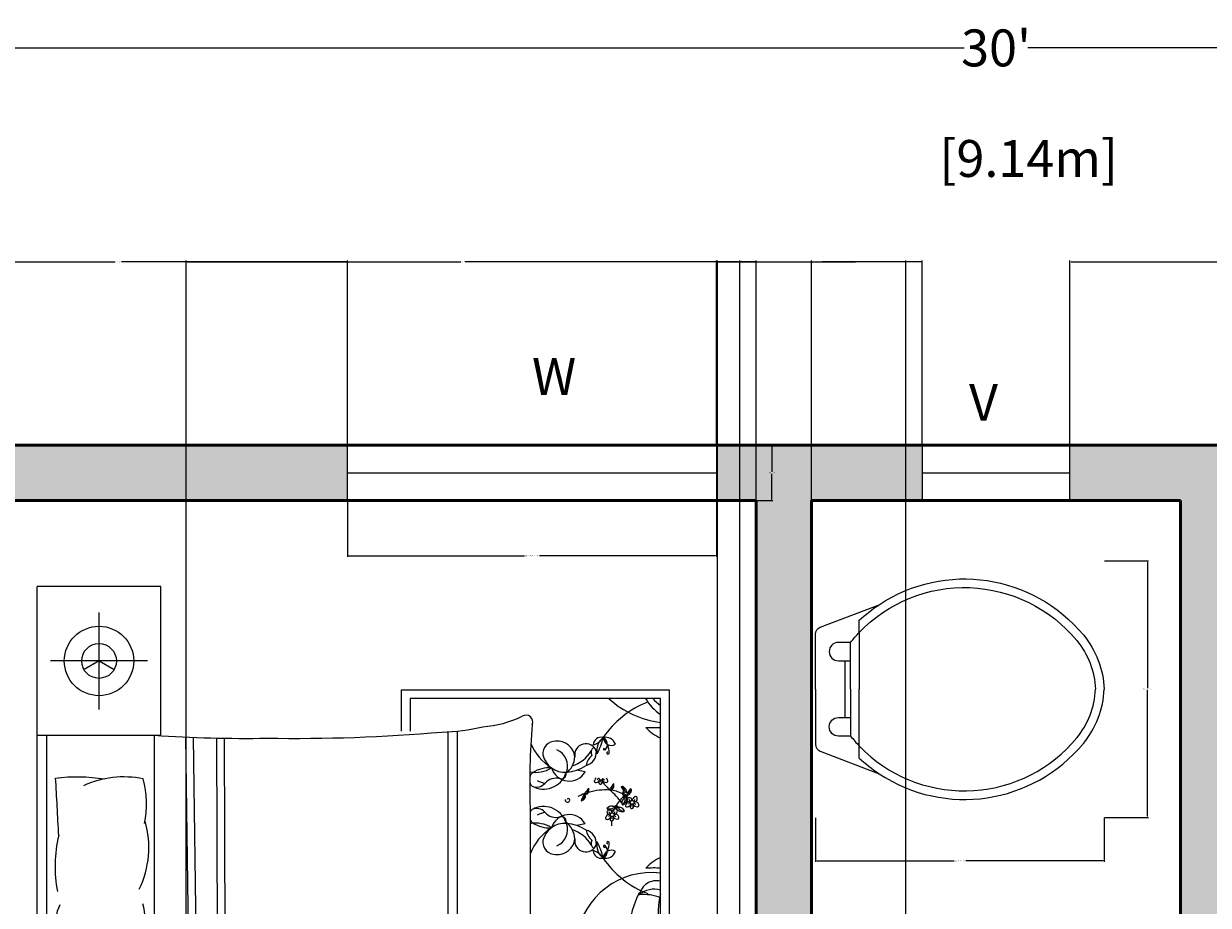
# Model space of a CAD drawing. Units: inches. Extents: x -55 to 413, y -498 to 86.
# Tile 5 of 6: x 45 to 238, y -57 to 86. Entities that reach past the tile are written whole.
import ezdxf

# ---------------------------------------------------------------- set-up
doc = ezdxf.new("R2010")
doc.units = ezdxf.units.IN
doc.header["$MEASUREMENT"] = 0
for name, color, linetype, lineweight in [('A-ANNO-DIMS', 2, 'Continuous', 18), ('A-ANNO-TEXT', 7, 'Continuous', 25), ('A-FLOR-FIXT', 9, 'Continuous', 18), ('A-FURN', 9, 'Continuous', 18), ('A-GLAZ', 4, 'Continuous', 18), ('A-WALL', 7, 'Continuous', 50), ('A-WALL-PATT', 8, 'Continuous', 13)]:
    doc.layers.add(name, color=color, linetype=linetype, lineweight=lineweight)
doc.styles.get("Standard").update_dxf_attribs({"font": 'arial.ttf'})
doc.dimstyles.get("Standard").update_dxf_attribs({"dimtxt": 0.18, "dimasz": 0.18, "dimexe": 0.18, "dimexo": 0.0625, "dimgap": 0.09, "dimtad": 0, "dimtih": 1, "dimtoh": 1, "dimdec": 0, "dimzin": 0, "dimdsep": 46, "dimlunit": 3, "dimtxsty": 'Standard', "dimcen": 0.09, "dimadec": 0, "dimazin": 0, "dimtfac": 1, "dimtdec": 0, "dimtofl": 0, "dimtmove": 0, "dimatfit": 3, "dimfxl": 1, "dimtolj": 1, "dimtzin": 0, "dimarcsym": 0})

# ---------------------------------------------------------------- blocks, each defined once
blk = doc.blocks.new('*D2')
at = {"layer": 'A-ANNO-DIMS', "color": 0, "lineweight": -2, "transparency": 16777216}
for p, q in [((23, 17.6), (23, 82.27)), ((23.18, 82.09), (197.82, 82.09)), ((382.82, 82.09), (208.18, 82.09)), ((383, 17.6), (383, 82.27))]:
    blk.add_line(p, q, dxfattribs=at)
at = {"layer": 'A-ANNO-DIMS', "color": 0, "transparency": 16777216}
for points in [[(23.18, 82.12), (23.18, 82.06), (23, 82.09)], [(382.82, 82.12), (382.82, 82.06), (383, 82.09)]]:
    blk.add_solid(points, dxfattribs=at)
at = {"layer": 'Defpoints', "color": 0, "transparency": 16777216}
for p in [(383, 82.09), (23, 17.54), (383, 17.54)]:
    blk.add_point(p, dxfattribs=at)
at = {"layer": 'A-ANNO-DIMS', "color": 0, "transparency": 16777216, "insert": (203, 82.09), "char_height": 6, "attachment_point": 5}
blk.add_mtext("\\A1;30'", dxfattribs=at)
blk = doc.blocks.new('BED-DOUBLE-WITH-NIGHTSTANDS')
for p, q in [((0, 0), (0, 120.84)), ((10.07, 100.86), (10.07, 116.65)), ((17.96, 108.75), (2.18, 108.75)), ((59.24, 97.34), (59.24, 104.05)), ((59.24, 104.05), (102.77, 104.05)), ((102.77, 104.05), (102.77, 15.95)), ((60.64, 102.65), (60.64, 97.32)), ((101.37, 102.65), (60.64, 102.65)), ((101.37, 17.35), (101.37, 102.65)), ((1.55, 96.67), (1.55, 24.17)), ((19.1, 24.17), (19.1, 96.67)), ((24.12, 96.35), (24.72, 53.32)), ((25.36, 96.3), (25.98, 52.42)), ((66.77, 97.22), (66.77, 22.78)), ((68.28, 97.33), (68.28, 22.78)), ((29.16, 96.24), (29.34, 50.35)), ((30.4, 96.24), (30.59, 49.88)), ((89.11, 90.74), (87.75, 91)), ((80.15, 84.95), (80.15, 35.89)), ((89.11, 82.29), (87.75, 82.03)), ((19.1, 57.36), (28.31, 50.74)), ((22.69, 40.95), (19.1, 54.13)), ((28.31, 50.74), (35.41, 48.05)), ((35.41, 48.05), (38.59, 47.56)), ((38.59, 47.56), (37.61, 43.64)), ((37.61, 43.64), (36.14, 40.46)), ((25.87, 32.14), (22.69, 40.95)), ((36.14, 40.46), (35.41, 35.08)), ((89.11, 37.7), (87.75, 37.97)), ((35.41, 35.08), (34.92, 28.96)), ((29.29, 27.49), (25.87, 32.14)), ((34.92, 28.96), (35.41, 24.06)), ((89.11, 29.26), (87.75, 28.99)), ((34.43, 23.09), (29.29, 27.49)), ((0, 24.17), (33.17, 24.17)), ((35.41, 24.06), (34.43, 23.09)), ((59.24, 15.95), (59.24, 22.78)), ((60.64, 22.78), (60.64, 17.35)), ((10.07, 19.98), (10.07, 4.19)), ((60.64, 17.35), (101.37, 17.35)), ((102.77, 15.95), (59.24, 15.95)), ((17.96, 12.08), (2.18, 12.08))]:
    blk.add_line(p, q)
for points in [[(0, 96.67), (20.14, 96.67), (20.14, 120.84), (0, 120.84)], [(10.07, 108.75), (7.63, 107.35)], [(10.07, 108.75), (12.51, 107.35)], [(20.14, 24.17), (20.14, 0), (0, 0)], [(10.07, 12.08), (7.63, 13.49)], [(10.07, 12.08), (12.51, 13.49)]]:
    blk.add_lwpolyline(points)
for points in [[(65.82, 97.19, 0.056112), (72.47, 98.06, 0.095341), (78.87, 99.76)], [(3.01, 89.73, -0.074897), (10.9, 89.58, 0.472817)], [(11.35, 65.01, -0.14099), (3.29, 64.77, -0.235245)], [(11.35, 59.85, 0.14099), (3.29, 60.09, 0.235245)], [(3.01, 31.11, 0.074897), (10.9, 31.25, -0.472817)], [(45.49, 22.83, 0.001242), (68.42, 22.78, -0.127202), (79.85, 20.35)]]:
    blk.add_lwpolyline(points, format="xyb")
for centre, radius in [((10.07, 108.75), 5.64), ((10.07, 108.75), 2.82), ((96.74, 85.77), 0.308), ((93.49, 83.76), 0.308), ((93.49, 36.24), 0.308), ((96.74, 34.23), 0.308), ((10.07, 12.08), 5.64), ((10.07, 12.08), 2.82)]:
    blk.add_circle(centre, radius)
for centre, radius, start, end in [((105.05, 87.4), 15.78, 111.4092, 145.6135), ((103.49, 114.39), 15.78, 228.1144, 262.255), ((105.6, 106.48), 7.69, 209.8884, 236.5383), ((107.04, 109.24), 9.58, 223.5186, 233.6964), ((79.49, 98.85), 1.1, 336.5219, 123.8264), ((197.68, 88.65), 117.59, 175.2402, 181.8035), ((33.86, 313.3), 217.13, 266.1, 270.9282), ((41.76, 379.4), 283.23, 269.1145, 274.8735), ((91.72, 95.04), 1.31, 76.272, 177.0484), ((89.73, 97.71), 2.7, 284.7031, 328.6173), ((93.49, 94.28), 2.49, 125.7657, 194.5347), ((81.25, 98.7), 11.04, 332.8176, 347.4827), ((92.4, 94.6), 1.75, 20.9613, 102.2885), ((93.35, 96.35), 1.32, 181.7131, 301.5367), ((89.03, 93.68), 3.99, 2.0648, 41.1598), ((91.43, 95.17), 1.29, 316.2238, 62.3173), ((103.83, 102.17), 6.42, 221.0454, 247.4453), ((100.38, 119.75), 21.83, 266.3481, 272.5919), ((88.66, 99), 9.15, 203.6453, 236.3329), ((84.27, 93.67), 2.04, 88.9462, 185.5144), ((84.56, 92.84), 2.89, 7.1143, 95.0551), ((89.21, 93.5), 1.81, 19.1312, 189.736), ((91.18, 93.88), 1.11, 126.7319, 206.0245), ((92.17, 94.41), 0.103, 20.2667, 316.2271), ((85.78, 94.3), 3.63, 193.079, 274.7067), ((83.46, 91.7), 2.8, 338.5779, 68.4181), ((83.92, 93.34), 3.51, 305.9599, 357.6409), ((85.22, 97.1), 5.7, 288.2955, 328.7386), ((88.67, 93.94), 2.26, 285.6955, 4.031), ((91.68, 91.5), 2.41, 128.4175, 173.8338), ((92.82, 93.82), 0.196, 168.5166, 2.0648), ((92.72, 93.84), 0.0952, 52.0591, 168.5166), ((81.49, 89.45), 1.46, 127.675, 162.5814), ((81.04, 95.65), 5.01, 259.249, 301.1782), ((83.22, 86.74), 4.66, 85.2696, 124.215), ((86.51, 92.24), 3, 196.8663, 330.0915), ((83.22, 86.74), 4.66, 53.6555, 57.2989), ((85.68, 97.15), 6.48, 273.4924, 303.7117), ((-1146.98, 23.12), 1151.92, 2.85022, 3.31479), ((14.07, 74.34), 15.57, 78.2417, 114.8684), ((1.6, 85.42), 16.19, 348.9631, 14.8961), ((81.49, 89.45), 1.46, 196.6343, 225.5483), ((82.34, 91.77), 3.85, 240.8249, 340.7178), ((81.2, 90.06), 1.81, 246.1646, 318.4347), ((83.04, 92.35), 3.47, 240.0851, 262.564), ((84.4, 87.22), 2.48, 74.8529, 138.4347), ((85.25, 90.33), 0.75, 254.8529, 12.6959), ((90.82, 89.21), 0.238, 125.0752, 284.7644), ((91.19, 89.3), 0.513, 127.3642, 168.4363), ((90.79, 89.71), 0.74, 277.4968, 341.2737), ((91.37, 89.36), 0.294, 88.1325, 178.8919), ((91.96, 89.05), 0.636, 136.3462, 189.6513), ((91.6, 88.99), 0.265, 189.6513, 312.3208), ((91.66, 89.72), 0.308, 183.2768, 356.7232), ((92.63, 89.17), 1.01, 164.2829, 186.9148), ((91.44, 89.17), 0.504, 312.3208, 40.2111), ((92.5, 89.73), 0.715, 201.6382, 274.947), ((91.56, 88.75), 0.934, 42.3896, 66.5724), ((100.98, 96.15), 11.47, 217.9541, 226.8459), ((92.23, 89.3), 0.508, 10.9597, 52.2379), ((92.55, 89.26), 0.236, 274.947, 37.5263), ((94.05, 88.22), 0.634, 115.5379, 168.6744), ((91.9, 89.14), 1.91, 329.344, 349.7412), ((90.37, 88.7), 3.41, 352.8698, 1.6736), ((92.47, 77.79), 10.01, 110.1059, 116.9968), ((86.93, 87.31), 1.94, 336.3901, 344.4871), ((89.04, 86.81), 0.246, 83.9457, 185.6216), ((88.06, 87.04), 1.01, 328.836, 0.8141), ((88.58, 86.75), 0.58, 306.5232, 32.4668), ((89.27, 87.2), 0.246, 112.5583, 214.2343), ((89.11, 87.64), 0.58, 265.7131, 351.6568), ((88.6, 87.96), 1.01, 297.3659, 329.344), ((87.84, 88.83), 1.94, 313.6929, 321.7899), ((89.98, 87.5), 0.634, 115.5379, 168.6744), ((87.83, 88.42), 1.91, 329.344, 349.7412), ((92.47, 77.79), 10.01, 86.1723, 106.4158), ((86.31, 87.98), 3.41, 352.8698, 1.6736), ((93.34, 87.92), 0.246, 112.5583, 214.2343), ((93.18, 88.36), 0.58, 265.7131, 351.6568), ((92.67, 88.68), 1.01, 297.3659, 329.344), ((92.72, 82.78), 5.02, 60.7959, 85.244), ((82.04, 75.56), 16.51, 37.8256, 47.7588), ((91.9, 89.55), 1.94, 313.6929, 321.7899), ((99.38, 82.26), 6.02, 130.182, 149.456), ((95.16, 88.01), 0.344, 33.0979, 123.1364), ((87.59, 83.16), 8.99, 31.1156, 34.8118), ((94.67, 87.42), 0.93, 2.3172, 70.5201), ((94.22, 86.41), 1.4, 310.9365, 22.7695), ((95.43, 87.19), 0.268, 135.7354, 318.1297), ((94.99, 87.63), 0.356, 315.7354, 31.1156), ((94.69, 86.87), 0.826, 319.3812, 5.5456), ((95.64, 87.19), 0.268, 68.2452, 250.6395), ((95.02, 87.52), 0.801, 352.6008, 57.1845), ((97.88, 82.14), 5.36, 111.7087, 116.2181), ((92.72, 82.78), 5.02, 47.5083, 55.9967), ((95.78, 87.7), 0.801, 252.8042, 349.6943), ((95.02, 86.27), 0.853, 331.1838, 51.6792), ((95.87, 87.77), 0.356, 248.2452, 323.6254), ((95.55, 87.99), 0.93, 291.7087, 3.0299), ((88.91, 92.89), 8.99, 323.6254, 327.3216), ((96.29, 87.75), 0.344, 325.6077, 55.6462), ((97.67, 85.85), 0.97, 121.9501, 165.2442), ((97.31, 86.42), 0.305, 44.3732, 121.9501), ((82.34, 81.26), 3.85, 19.2822, 119.1751), ((81.2, 82.97), 1.81, 41.5653, 113.8354), ((86.24, 86.19), 0.379, 169.5864, 349.5616), ((86.38, 86.17), 0.233, 349.5616, 167.2949), ((89.11, 86.04), 0.634, 129.5056, 182.6421), ((87.29, 87.51), 1.91, 308.4388, 328.836), ((86.96, 89.06), 3.41, 296.5064, 305.3102), ((93.04, 86.11), 1.4, 253.6301, 325.4631), ((93.43, 84.17), 0.992, 82.0748, 142.6895), ((93.32, 85.53), 1.02, 228.342, 274.9894), ((93.35, 85.36), 0.853, 273.8774, 357.1501), ((93.68, 85.97), 0.826, 262.0748, 308.2393), ((95.01, 85.12), 0.853, 181.4625, 249.4747), ((94.87, 85.79), 0.826, 215.1128, 261.2773), ((95.53, 85.75), 1.4, 197.889, 269.722), ((94.59, 84), 0.992, 20.6625, 81.2773), ((96.07, 85.69), 0.992, 139.3812, 199.9959), ((94.86, 86.33), 1.02, 285.6484, 332.2957), ((95.89, 85.25), 0.238, 125.0752, 284.7644), ((96.26, 85.34), 0.513, 93.635, 168.4363), ((96.19, 86.16), 0.302, 138.2946, 276.2474), ((95.86, 85.76), 0.74, 277.4968, 341.2737), ((96.31, 86.11), 0.42, 358.5719, 143.8954), ((96.45, 85.41), 0.294, 88.1325, 178.8919), ((96.55, 86.44), 0.424, 208.8493, 269.9355), ((96.19, 86.34), 0.484, 274.2123, 318.1587), ((97.04, 85.1), 0.636, 136.3462, 189.6513), ((96.67, 85.04), 0.265, 189.6513, 312.3208), ((97.7, 85.22), 1.01, 164.2829, 186.9148), ((96.51, 85.21), 0.504, 312.3208, 40.2111), ((97.58, 85.78), 0.715, 201.6382, 274.947), ((97, 86.23), 0.204, 262.868, 7.094), ((96.63, 84.8), 0.934, 42.3896, 66.5724), ((96.97, 86.4), 0.607, 278.5614, 22.5914), ((97.31, 85.35), 0.508, 10.9597, 118.7804), ((97.62, 85.3), 0.236, 274.947, 37.5263), ((81.49, 83.58), 1.46, 134.4517, 156.7144), ((81.49, 83.58), 1.46, 203.2856, 232.325), ((83.04, 80.68), 3.47, 97.436, 119.9149), ((84.4, 85.81), 2.48, 221.5653, 285.1471), ((86.51, 80.79), 3, 29.9085, 163.1337), ((85.25, 82.7), 0.75, 347.3041, 105.1471), ((92.65, 83.24), 0.238, 125.0752, 284.7644), ((93.02, 83.33), 0.513, 93.635, 168.4363), ((92.95, 84.14), 0.302, 138.2946, 276.2474), ((92.61, 83.74), 0.74, 277.4968, 341.2737), ((93.06, 84.1), 0.42, 358.5719, 143.8954), ((93.2, 83.4), 0.294, 88.1325, 178.8919), ((93.31, 84.43), 0.424, 208.8493, 269.9355), ((92.95, 84.33), 0.484, 274.2123, 318.1587), ((93.79, 83.09), 0.636, 136.3462, 189.6513), ((93.43, 83.02), 0.265, 189.6513, 312.3208), ((94.45, 83.21), 1.01, 164.2829, 186.9148), ((94.42, 83.84), 0.97, 121.9501, 165.2442), ((93.27, 83.2), 0.504, 312.3208, 40.2111), ((94.33, 83.77), 0.715, 201.6382, 274.947), ((93.75, 84.21), 0.204, 262.868, 7.094), ((93.39, 82.79), 0.934, 42.3896, 66.5724), ((93.73, 84.38), 0.607, 278.5614, 22.5914), ((94.06, 83.34), 0.508, 10.9597, 118.7804), ((99.38, 82.26), 6.02, 156.1523, 156.9499), ((94.07, 84.4), 0.305, 44.3732, 121.9501), ((94.37, 83.29), 0.236, 274.947, 37.5263), ((95.09, 85.27), 1.02, 248.3627, 295.0101), ((2.79, 78.43), 15.38, 333.8761, 16.1746), ((81.04, 77.38), 5.01, 58.8218, 100.2867), ((88.66, 74.03), 9.15, 123.6671, 158.5059), ((83.22, 86.29), 4.66, 235.785, 274.7304), ((85.78, 78.73), 3.63, 85.2933, 166.921), ((83.46, 81.33), 2.8, 291.5819, 21.4221), ((83.22, 86.29), 4.66, 302.7011, 306.3445), ((83.92, 79.69), 3.51, 2.3591, 54.0401), ((85.68, 75.88), 6.48, 56.2883, 86.5076), ((85.22, 75.93), 5.7, 31.2614, 71.7045), ((91.68, 81.53), 2.41, 186.1662, 231.5825), ((88.67, 79.09), 2.26, 355.969, 74.3045), ((99.38, 82.26), 6.02, 175.2415, 182.8929), ((24.16, 75.39), 21.24, 166.3427, 191.1841), ((84.27, 79.36), 2.04, 174.4856, 271.0538), ((84.56, 80.19), 2.89, 264.9449, 352.8857), ((89.21, 79.53), 1.81, 170.264, 340.8688), ((91.18, 79.16), 1.11, 153.9755, 233.2681), ((93.49, 78.75), 2.49, 165.4653, 234.2343), ((81.25, 74.33), 11.04, 12.5173, 27.1824), ((89.03, 79.35), 3.99, 318.8402, 357.9352), ((92.82, 79.21), 0.196, 357.9352, 191.4834), ((92.72, 79.19), 0.0952, 191.4834, 307.9409), ((91.72, 77.99), 1.31, 182.9516, 283.728), ((89.73, 75.32), 2.7, 31.3827, 75.2969), ((91.43, 77.86), 1.29, 297.6827, 43.7762), ((93.35, 76.68), 1.32, 58.4633, 178.2869), ((92.4, 78.43), 1.75, 257.7115, 339.0387), ((92.24, 78.64), 0.171, 43.7762, 339.7183), ((105.05, 85.63), 15.78, 214.3865, 248.5908), ((103.83, 70.86), 6.42, 112.5547, 138.9546), ((100.38, 53.28), 21.83, 87.4081, 93.6519), ((99.85, 62.15), 12.21, 82.8636, 171.8197), ((100.7, 70.21), 2.83, 76.3898, 169.0739), ((100.31, 68.09), 3.58, 72.8609, 131.9049), ((111.94, 63.87), 15.78, 152.5854, 175.5377), ((98.73, 63.73), 7.06, 68.117, 96.6195), ((109.66, 68.29), 8.68, 162.9798, 196.4569), ((9.04, 66.43), 5.98, 153.3437, 196.1026), ((11.12, 67.24), 6.41, 335.0183, 18.5407), ((97.39, 63.8), 1.75, 50.8855, 132.2127), ((114.13, 64.85), 12.83, 174.3643, 175.6213), ((122.92, 58.09), 22.93, 160.0972, 160.2783), ((15.38, 79.26), 14.81, 254.1707, 275.9871), ((88.12, 62.64), 1.31, 106.1963, 206.9726), ((85.07, 63.96), 2.7, 314.6273, 358.5415), ((90.03, 62.87), 2.49, 155.6899, 224.4589), ((88.94, 62.6), 1.75, 50.8855, 132.2127), ((88.88, 64.58), 1.32, 211.6373, 331.4609), ((87.81, 62.6), 1.29, 346.148, 92.2415), ((86.47, 60.12), 3.99, 31.989, 71.0841), ((77.23, 60.59), 11.04, 2.7418, 17.407), ((96.58, 63.84), 1.31, 106.1963, 206.9726), ((93.52, 65.17), 2.7, 314.6273, 358.5415), ((98.49, 64.07), 2.49, 155.6899, 224.4589), ((97.33, 65.79), 1.32, 211.6373, 331.4609), ((94.92, 61.33), 3.99, 31.989, 71.0841), ((85.68, 61.8), 11.04, 2.7418, 17.407), ((96.26, 63.81), 1.29, 346.148, 92.2415), ((97.28, 63.53), 0.103, 50.1909, 346.0209), ((88.12, 61.39), 1.31, 153.0274, 253.8037), ((85.07, 60.06), 2.7, 1.4585, 45.3727), ((90.03, 61.16), 2.49, 135.5411, 204.3101), ((77.23, 63.43), 11.04, 342.593, 357.2582), ((86.47, 63.91), 3.99, 288.9159, 328.011), ((87.81, 61.42), 1.29, 267.7585, 13.852), ((88.83, 62.32), 0.103, 50.1909, 346.0209), ((88.9, 61.69), 0.171, 13.852, 309.9245), ((89.59, 62.1), 0.0952, 81.9833, 198.4408), ((89.59, 61.93), 0.0952, 161.5592, 278.0167), ((89.68, 62.13), 0.196, 198.4408, 31.989), ((89.68, 61.9), 0.196, 328.011, 161.5592), ((98.49, 59.95), 2.49, 135.5411, 204.3101), ((85.68, 62.23), 11.04, 342.593, 357.2582), ((98.14, 63.34), 0.196, 198.4408, 31.989), ((98.04, 63.3), 0.0952, 81.9833, 198.4408), ((24.59, 56.92), 21.53, 171.5249, 193.96), ((15.38, 45.61), 14.81, 84.0129, 105.8293), ((-3.78, 55.31), 21.31, 349.8617, 13.6238), ((88.88, 59.44), 1.32, 28.5391, 148.3627), ((88.94, 61.43), 1.75, 227.7873, 309.1145), ((103.49, 61.36), 15.78, 184.4623, 262.255), ((96.58, 60.18), 1.31, 153.0274, 253.8037), ((93.52, 58.85), 2.7, 1.4585, 45.3727), ((94.92, 62.7), 3.99, 288.9159, 328.011), ((96.26, 60.21), 1.29, 267.7585, 13.852), ((97.35, 60.48), 0.171, 13.852, 309.9245), ((98.14, 60.69), 0.196, 328.011, 161.5592), ((98.04, 60.72), 0.0952, 161.5592, 278.0167), ((97.33, 58.23), 1.32, 28.5391, 148.3627), ((97.39, 60.22), 1.75, 227.7873, 309.1145), ((111.94, 60.15), 15.78, 184.4623, 207.4146), ((109.66, 55.74), 8.68, 163.5431, 197.0202), ((114.13, 59.18), 12.83, 184.3787, 185.6357), ((122.92, 65.93), 22.93, 199.7217, 199.9028), ((46.74, 47.67), 43.83, 172.2196, 189.497), ((-9.91, 43.94), 28.09, 348.0397, 19.2615), ((105.6, 53.44), 7.69, 181.272, 236.5383), ((109.73, 61.24), 14.25, 214.0123, 234.053), ((107.04, 56.21), 9.58, 197.8504, 233.6964), ((105.05, 34.36), 15.78, 111.4092, 145.6135), ((-7.08, 55.95), 46.86, 340.1194, 349.3383), ((38.69, 47.29), 0.292, 358.8623, 109.7536), ((100.38, 66.71), 21.83, 266.3481, 272.5919), ((103.83, 49.14), 6.42, 221.0454, 247.4453), ((88.66, 45.97), 9.15, 201.4941, 236.3329), ((84.27, 40.64), 2.04, 88.9462, 185.5144), ((84.56, 39.8), 2.89, 7.1143, 95.0551), ((91.72, 42), 1.31, 76.272, 177.0484), ((89.73, 44.68), 2.7, 284.7031, 328.6173), ((93.49, 41.25), 2.49, 125.7657, 194.5347), ((81.25, 45.67), 11.04, 332.8176, 347.4827), ((92.4, 41.56), 1.75, 20.9613, 102.2885), ((91.43, 42.13), 1.29, 316.2238, 62.3173), ((89.03, 40.65), 3.99, 2.0648, 41.1598), ((93.35, 43.31), 1.32, 181.7131, 301.5367), ((83.46, 38.67), 2.8, 338.5779, 68.4181), ((85.22, 44.06), 5.7, 288.2955, 328.7386), ((89.21, 40.47), 1.81, 19.1312, 189.736), ((88.67, 40.9), 2.26, 285.6955, 4.031), ((91.18, 40.84), 1.11, 126.7319, 206.0245), ((92.17, 41.37), 0.103, 20.2667, 316.2271), ((92.82, 40.78), 0.196, 168.5166, 2.0648), ((92.72, 40.8), 0.0952, 52.0591, 168.5166), ((-1146.98, 97.71), 1151.92, 356.68521, 357.14978), ((1.6, 35.42), 16.19, 345.1039, 11.0369), ((46, 36.05), 9.84, 156.2616, 191.3392), ((85.78, 41.27), 3.63, 193.079, 274.7067), ((83.92, 40.3), 3.51, 305.9599, 357.6409), ((85.68, 44.12), 6.48, 273.4924, 303.7117), ((91.68, 38.46), 2.41, 128.4175, 173.8338), ((81.04, 42.61), 5.01, 259.7133, 301.1782), ((81.49, 36.41), 1.46, 127.675, 156.7144), ((82.34, 38.74), 3.85, 240.8249, 340.7178), ((83.22, 33.71), 4.66, 85.2696, 124.215), ((84.4, 34.18), 2.48, 74.8529, 138.4347), ((86.51, 39.2), 3, 196.8663, 330.0915), ((85.25, 37.3), 0.75, 254.8529, 12.6959), ((83.22, 33.71), 4.66, 53.6555, 57.2989), ((92.65, 36.76), 0.238, 75.2356, 234.9248), ((92.61, 36.25), 0.74, 18.7263, 82.5032), ((93.2, 36.6), 0.294, 181.1081, 271.8675), ((93.79, 36.91), 0.636, 170.3487, 223.6538), ((93.43, 36.97), 0.265, 47.6792, 170.3487), ((99.38, 37.73), 6.02, 177.1071, 184.7585), ((94.45, 36.79), 1.01, 173.0852, 195.7171), ((93.27, 36.8), 0.504, 319.7889, 47.6792), ((94.33, 36.23), 0.715, 85.053, 158.3618), ((94.37, 36.71), 0.236, 322.4737, 85.053), ((205.94, 34.45), 125.79, 179.3433, 185.6887), ((81.49, 36.41), 1.46, 203.229, 225.5483), ((81.2, 37.03), 1.81, 246.1646, 318.4347), ((83.04, 39.32), 3.47, 240.0851, 262.564), ((93.02, 36.66), 0.513, 191.5637, 266.365), ((93.32, 34.47), 1.02, 85.0106, 131.658), ((93.04, 33.88), 1.4, 34.5369, 106.3699), ((93.43, 35.83), 0.992, 217.3105, 277.9252), ((92.95, 35.85), 0.302, 83.7526, 221.7054), ((93.06, 35.9), 0.42, 216.1046, 1.4281), ((93.31, 35.57), 0.424, 90.0645, 151.1507), ((92.95, 35.67), 0.484, 41.8413, 85.7877), ((93.35, 34.63), 0.853, 2.8499, 86.1226), ((94.42, 36.16), 0.97, 194.7558, 238.0499), ((93.68, 34.03), 0.826, 51.7607, 97.9252), ((93.75, 35.78), 0.204, 352.906, 97.132), ((93.39, 37.21), 0.934, 293.4276, 317.6104), ((94.06, 36.66), 0.508, 241.2196, 349.0403), ((93.73, 35.61), 0.607, 337.4086, 81.4386), ((99.38, 37.73), 6.02, 203.0501, 203.8477), ((94.07, 35.59), 0.305, 238.0499, 315.6268), ((95.01, 34.88), 0.853, 110.5253, 178.5375), ((95.53, 34.25), 1.4, 90.278, 162.111), ((94.87, 34.2), 0.826, 98.7227, 144.8872), ((99.38, 37.73), 6.02, 210.544, 229.818), ((95.09, 34.73), 1.02, 64.9899, 111.6373), ((94.59, 36), 0.992, 278.7227, 339.3375), ((95.89, 34.74), 0.238, 75.2356, 234.9248), ((95.86, 34.24), 0.74, 18.7263, 82.5032), ((97.04, 34.9), 0.636, 170.3487, 223.6538), ((96.67, 34.96), 0.265, 47.6792, 170.3487), ((97.7, 34.78), 1.01, 173.0852, 195.7171), ((96.51, 34.78), 0.504, 319.7889, 47.6792), ((97.58, 34.22), 0.715, 85.053, 158.3618), ((97.62, 34.69), 0.236, 322.4737, 85.053), ((-8.36, 25.15), 45.61, 357.4519, 11.3392), ((86.24, 33.8), 0.379, 10.4384, 190.4136), ((86.38, 33.83), 0.233, 192.7051, 10.4384), ((92.47, 42.2), 10.01, 243.0032, 249.8941), ((87.29, 32.49), 1.91, 31.164, 51.5612), ((89.11, 33.95), 0.634, 177.3579, 230.4944), ((86.96, 30.93), 3.41, 54.6898, 63.4936), ((86.93, 32.69), 1.94, 15.5129, 23.6099), ((89.04, 33.18), 0.246, 174.3784, 276.0543), ((88.06, 32.95), 1.01, 359.1859, 31.164), ((88.58, 33.25), 0.58, 327.5332, 53.4768), ((89.27, 32.8), 0.246, 145.7657, 247.4417), ((89.11, 32.36), 0.58, 8.3432, 94.2869), ((88.6, 32.04), 1.01, 30.656, 62.6341), ((82.04, 44.44), 16.51, 312.2412, 322.1744), ((92.72, 37.22), 5.02, 274.756, 299.2041), ((96.07, 34.31), 0.992, 160.0041, 220.6188), ((94.22, 33.59), 1.4, 337.2305, 49.0635), ((94.86, 33.66), 1.02, 27.7043, 74.3516), ((95.43, 32.81), 0.268, 41.8703, 224.2646), ((94.69, 33.12), 0.826, 354.4544, 40.6188), ((95.64, 32.8), 0.268, 109.3605, 291.7548), ((97.88, 37.85), 5.36, 243.7819, 248.2913), ((92.72, 37.22), 5.02, 304.0033, 312.4917), ((95.02, 33.73), 0.853, 308.3208, 28.8162), ((95.78, 32.29), 0.801, 10.3057, 107.1958), ((96.26, 34.65), 0.513, 191.5637, 266.365), ((96.19, 33.84), 0.302, 83.7526, 221.7054), ((95.55, 32.01), 0.93, 356.9701, 68.2913), ((96.31, 33.89), 0.42, 216.1046, 1.4281), ((96.45, 34.58), 0.294, 181.1081, 271.8675), ((96.55, 33.56), 0.424, 90.0645, 151.1507), ((96.19, 33.66), 0.484, 41.8413, 85.7877), ((97.67, 34.14), 0.97, 194.7558, 238.0499), ((97, 33.77), 0.204, 352.906, 97.132), ((96.63, 35.19), 0.934, 293.4276, 317.6104), ((97.31, 34.65), 0.508, 241.2196, 349.0403), ((96.97, 33.6), 0.607, 337.4086, 81.4386), ((97.31, 33.58), 0.305, 238.0499, 315.6268), ((14.07, 46.5), 15.57, 245.1316, 281.7583), ((81.49, 30.55), 1.46, 134.4517, 153.558), ((82.34, 28.23), 3.85, 19.2822, 119.1751), ((81.2, 29.93), 1.81, 41.5653, 113.8354), ((83.04, 27.64), 3.47, 97.436, 119.9149), ((84.4, 32.78), 2.48, 221.5653, 285.1471), ((87.84, 31.17), 1.94, 38.2101, 46.3071), ((89.98, 32.49), 0.634, 191.3256, 244.4621), ((87.83, 31.58), 1.91, 10.2588, 30.656), ((92.47, 42.2), 10.01, 253.5842, 273.8277), ((86.31, 32.02), 3.41, 358.3264, 7.1302), ((90.82, 30.79), 0.238, 75.2356, 234.9248), ((90.79, 30.29), 0.74, 18.7263, 82.5032), ((91.96, 30.94), 0.636, 170.3487, 223.6538), ((91.6, 31.01), 0.265, 47.6792, 170.3487), ((92.63, 30.82), 1.01, 173.0852, 195.7171), ((91.44, 30.83), 0.504, 319.7889, 47.6792), ((92.5, 30.26), 0.715, 85.053, 158.3618), ((100.98, 23.85), 11.47, 133.1541, 142.0459), ((92.55, 30.74), 0.236, 322.4737, 85.053), ((93.34, 32.08), 0.246, 145.7657, 247.4417), ((93.18, 31.64), 0.58, 8.3432, 94.2869), ((92.67, 31.32), 1.01, 30.656, 62.6341), ((91.9, 30.45), 1.94, 38.2101, 46.3071), ((94.05, 31.77), 0.634, 191.3256, 244.4621), ((91.9, 30.86), 1.91, 10.2588, 30.656), ((90.37, 31.3), 3.41, 358.3264, 7.1302), ((94.67, 32.58), 0.93, 289.4799, 357.6828), ((87.59, 36.83), 8.99, 325.1882, 328.8844), ((95.16, 31.99), 0.344, 236.8636, 326.9021), ((94.99, 32.37), 0.356, 328.8844, 44.2646), ((95.02, 32.47), 0.801, 302.8155, 7.3992), ((95.87, 32.22), 0.356, 36.3746, 111.7548), ((88.91, 27.1), 8.99, 32.6784, 36.3746), ((96.29, 32.24), 0.344, 304.3538, 34.3923), ((81.49, 30.55), 1.46, 210.0293, 232.325), ((81.04, 24.35), 5.01, 58.8218, 99.1554), ((83.22, 33.25), 4.66, 235.785, 274.7304), ((85.78, 25.7), 3.63, 85.2933, 166.921), ((86.51, 27.76), 3, 29.9085, 163.1337), ((83.46, 28.29), 2.8, 291.5819, 21.4221), ((85.25, 29.66), 0.75, 347.3041, 105.1471), ((83.22, 33.25), 4.66, 302.7011, 306.3445), ((83.92, 26.66), 3.51, 2.3591, 54.0401), ((85.68, 22.84), 6.48, 56.2883, 86.5076), ((91.19, 30.7), 0.513, 191.5637, 232.6358), ((91.37, 30.63), 0.294, 181.1081, 271.8675), ((91.66, 30.27), 0.308, 3.2768, 176.7232), ((91.56, 31.24), 0.934, 293.4276, 317.6104), ((92.23, 30.69), 0.508, 307.7621, 349.0403), ((88.66, 20.99), 9.15, 123.6671, 153.2997), ((85.22, 22.9), 5.7, 31.2614, 71.7045), ((88.67, 26.06), 2.26, 355.969, 74.3045), ((91.68, 28.5), 2.41, 186.1662, 231.5825), ((84.27, 26.32), 2.04, 174.4856, 271.0538), ((84.56, 27.16), 2.89, 264.9449, 352.8857), ((89.21, 26.49), 1.81, 170.264, 340.8688), ((91.18, 26.12), 1.11, 153.9755, 233.2681), ((93.49, 25.71), 2.49, 165.4653, 234.2343), ((81.25, 21.29), 11.04, 12.5173, 27.1824), ((89.03, 26.31), 3.99, 318.8402, 357.9352), ((91.43, 24.83), 1.29, 297.6827, 43.7762), ((92.24, 25.6), 0.171, 43.7762, 339.7183), ((92.82, 26.18), 0.196, 357.9352, 191.4834), ((92.72, 26.16), 0.0952, 191.4834, 307.9409), ((37.43, -87.71), 110.84, 85.8294, 91.553), ((89.73, 22.28), 2.7, 31.3827, 75.2969), ((91.72, 24.96), 1.31, 182.9516, 283.728), ((93.35, 23.65), 1.32, 58.4633, 178.2869), ((92.4, 25.4), 1.75, 257.7115, 339.0387), ((105.05, 32.6), 15.78, 214.3865, 248.5908), ((103.83, 17.82), 6.42, 112.5547, 138.9546), ((79.77, 21.46), 1.11, 273.98, 27.3412), ((103.49, 5.6), 15.78, 97.745, 131.8856), ((100.38, 0.25), 21.83, 87.4081, 93.6519), ((105.6, 13.52), 7.69, 123.4617, 150.1116), ((107.04, 10.75), 9.58, 126.3036, 136.4814)]:
    blk.add_arc(centre, radius, start, end)
blk = doc.blocks.new('WC-PLAN')
for p, q in [((7.1, 27.15), (7.1, 29.12)), ((7.1, 27.15), (7.1, 17.92)), ((7.1, 8.69), (7.1, 17.92)), ((7.1, 6.73), (7.1, 8.69))]:
    blk.add_line(p, q)
for points in [[(10.32, 31.66, -0.383919), (43.53, 26.74, -0.163732), (46.92, 17.92, -0.359733)], [(7.1, 27.15, -0.448546), (42.45, 25.85, -0.162618), (45.51, 17.92, -0.470877)], [(0, 17.92), (0, 26.88, -0.31031), (0.75, 27.98), (10.32, 31.66, -0.209071)], [(7.1, 29.12, -0.040937), (10.32, 31.66, -0.163732)], [(5.69, 25.54, -0.022712), (7.1, 27.15, -0.162618)], [(5.69, 25.54), (3.72, 25.54, 1), (3.72, 22.54), (4.74, 22.54)], [(5.69, 17.92), (5.69, 25.54, -0.476108)], [(0, 17.92), (0, 8.97, 0.31031), (0.75, 7.87), (10.32, 4.19, 0.209071)], [(5.69, 17.92), (5.69, 10.31, 0.022712)], [(8.06, 7.75, 0.431639), (42.45, 10, 0.162618), (45.51, 17.92, 0.470877)], [(10.32, 4.19, 0.383919), (43.53, 9.11, 0.163732), (46.92, 17.92, 0.359733)], [(5.69, 10.31), (3.72, 10.31, -1), (3.72, 13.31), (4.74, 13.31)], [(5.69, 10.31, 0.022712), (7.1, 8.69, 0.162618)], [(7.1, 8.69, 0.014165), (8.06, 7.75, 0.162618)], [(7.1, 6.73, 0.040937), (10.32, 4.19, 0.163732)]]:
    blk.add_lwpolyline(points, format="xyb")
for points in [[(4.74, 22.54), (4.74, 13.31)], [(4.74, 22.54), (5.69, 22.54)], [(4.74, 13.31), (5.69, 13.31)]]:
    blk.add_lwpolyline(points)
blk = doc.blocks.new('WIN-60IN')
for p, q in [((0, 9), (60, 9)), ((0, 0), (0, 9)), ((60, 9), (60, 0)), ((0, 4.5), (60, 4.5)), ((60, 0), (0, 0))]:
    blk.add_line(p, q)
blk = doc.blocks.new('WIN-24IN')
for p, q in [((24, 9), (0, 9)), ((0, 9), (0, 0)), ((24, 0), (24, 9)), ((0, 4.5), (24, 4.5)), ((0, 0), (24, 0))]:
    blk.add_line(p, q)
blk = doc.blocks.new('*D11')
at = {"layer": 'A-ANNO-DIMS', "color": 0, "lineweight": -2, "transparency": 16777216}
for p, q in [((97.55, 8.48), (97.55, -0.64)), ((157.55, 8.48), (157.55, -0.64)), ((97.73, -0.46), (126.32, -0.46)), ((157.37, -0.46), (128.78, -0.46))]:
    blk.add_line(p, q, dxfattribs=at)
at = {"layer": 'A-ANNO-DIMS', "color": 0, "transparency": 16777216}
for points in [[(97.73, -0.43), (97.73, -0.49), (97.55, -0.46)], [(157.37, -0.43), (157.37, -0.49), (157.55, -0.46)]]:
    blk.add_solid(points, dxfattribs=at)
at = {"layer": 'Defpoints', "color": 0, "transparency": 16777216}
for p in [(97.55, 8.54), (157.55, 8.54), (157.55, -0.46)]:
    blk.add_point(p, dxfattribs=at)
at = {"layer": 'A-ANNO-DIMS', "color": 0, "transparency": 16777216, "insert": (127.55, -0.46), "char_height": 0.18, "attachment_point": 5}
blk.add_mtext('\\A1;WINDOW 5\'-0" TYP.', dxfattribs=at)
blk = doc.blocks.new('*D12')
at = {"layer": 'A-ANNO-DIMS', "color": 0, "lineweight": -2, "transparency": 16777216}
for p, q in [((157.62, 17.54), (166.73, 17.54)), ((166.55, 17.36), (166.55, 13.22)), ((166.55, 8.72), (166.55, 12.86)), ((157.62, 8.54), (166.73, 8.54))]:
    blk.add_line(p, q, dxfattribs=at)
at = {"layer": 'A-ANNO-DIMS', "color": 0, "transparency": 16777216}
for points in [[(166.52, 17.36), (166.58, 17.36), (166.55, 17.54)], [(166.52, 8.72), (166.58, 8.72), (166.55, 8.54)]]:
    blk.add_solid(points, dxfattribs=at)
at = {"layer": 'Defpoints', "color": 0, "transparency": 16777216}
for p in [(157.55, 17.54), (166.55, 17.54), (157.55, 8.54)]:
    blk.add_point(p, dxfattribs=at)
at = {"layer": 'A-ANNO-DIMS', "color": 0, "transparency": 16777216, "insert": (166.55, 13.04), "char_height": 0.18, "attachment_point": 5}
blk.add_mtext('\\A1;0\'-9" TYP.', dxfattribs=at)
blk = doc.blocks.new('*D21')
at = {"layer": 'A-ANNO-DIMS', "color": 0, "lineweight": -2, "transparency": 16777216}
for p, q in [((173.66, -43.02), (173.66, -50.18)), ((220.58, -43.02), (220.58, -50.18)), ((173.84, -50), (196.17, -50)), ((220.4, -50), (198.08, -50))]:
    blk.add_line(p, q, dxfattribs=at)
at = {"layer": 'A-ANNO-DIMS', "color": 0, "transparency": 16777216}
for points in [[(173.84, -49.97), (173.84, -50.03), (173.66, -50)], [(220.4, -49.97), (220.4, -50.03), (220.58, -50)]]:
    blk.add_solid(points, dxfattribs=at)
at = {"layer": 'Defpoints', "color": 0, "transparency": 16777216}
for p in [(173.66, -42.96), (220.58, -42.96), (220.58, -50)]:
    blk.add_point(p, dxfattribs=at)
at = {"layer": 'A-ANNO-DIMS', "color": 0, "transparency": 16777216, "insert": (197.12, -50), "char_height": 0.18, "attachment_point": 5}
blk.add_mtext('\\A1;WC 3\'-11" TYP.', dxfattribs=at)
blk = doc.blocks.new('*D22')
at = {"layer": 'A-ANNO-DIMS', "color": 0, "lineweight": -2, "transparency": 16777216}
for p, q in [((220.64, -1.28), (227.8, -1.28)), ((227.62, -1.46), (227.62, -21.94)), ((227.62, -42.78), (227.62, -22.3)), ((220.64, -42.96), (227.8, -42.96))]:
    blk.add_line(p, q, dxfattribs=at)
at = {"layer": 'A-ANNO-DIMS', "color": 0, "transparency": 16777216}
for points in [[(227.59, -1.46), (227.65, -1.46), (227.62, -1.28)], [(227.59, -42.78), (227.65, -42.78), (227.62, -42.96)]]:
    blk.add_solid(points, dxfattribs=at)
at = {"layer": 'Defpoints', "color": 0, "transparency": 16777216}
for p in [(220.58, -1.28), (227.62, -1.28), (220.58, -42.96)]:
    blk.add_point(p, dxfattribs=at)
at = {"layer": 'A-ANNO-DIMS', "color": 0, "transparency": 16777216, "insert": (227.62, -22.12), "char_height": 0.18, "attachment_point": 5}
blk.add_mtext('\\A1;3\'-5 1/2" TYP.', dxfattribs=at)
blk = doc.blocks.new('*D27')
at = {"layer": 'A-ANNO-DIMS', "color": 0, "lineweight": -2, "transparency": 16777216}
for p, q in [((23, 17.6), (23, 47.52)), ((23.18, 47.34), (59.74, 47.34)), ((97.37, 47.34), (60.82, 47.34)), ((97.55, 17.6), (97.55, 47.52))]:
    blk.add_line(p, q, dxfattribs=at)
at = {"layer": 'A-ANNO-DIMS', "color": 0, "transparency": 16777216}
for points in [[(23.18, 47.37), (23.18, 47.31), (23, 47.34)], [(97.37, 47.37), (97.37, 47.31), (97.55, 47.34)]]:
    blk.add_solid(points, dxfattribs=at)
at = {"layer": 'Defpoints', "color": 0, "transparency": 16777216}
for p in [(97.55, 47.34), (23, 17.54), (97.55, 17.54)]:
    blk.add_point(p, dxfattribs=at)
at = {"layer": 'A-ANNO-DIMS', "color": 0, "transparency": 16777216, "insert": (60.28, 47.34), "char_height": 0.18, "attachment_point": 5}
blk.add_mtext('\\A1;6\'-2 1/2"', dxfattribs=at)
blk = doc.blocks.new('*D28')
at = {"layer": 'A-ANNO-DIMS', "color": 0, "lineweight": -2, "transparency": 16777216}
for p, q in [((157.55, 17.6), (157.55, 47.52)), ((157.73, 47.34), (173.74, 47.34)), ((190.82, 47.34), (174.82, 47.34)), ((191, 17.6), (191, 47.52))]:
    blk.add_line(p, q, dxfattribs=at)
at = {"layer": 'A-ANNO-DIMS', "color": 0, "transparency": 16777216}
for points in [[(157.73, 47.37), (157.73, 47.31), (157.55, 47.34)], [(190.82, 47.37), (190.82, 47.31), (191, 47.34)]]:
    blk.add_solid(points, dxfattribs=at)
at = {"layer": 'Defpoints', "color": 0, "transparency": 16777216}
for p in [(191, 47.34), (157.55, 17.54), (191, 17.54)]:
    blk.add_point(p, dxfattribs=at)
at = {"layer": 'A-ANNO-DIMS', "color": 0, "transparency": 16777216, "insert": (174.28, 47.34), "char_height": 0.18, "attachment_point": 5}
blk.add_mtext('\\A1;2\'-9 1/2"', dxfattribs=at)
blk = doc.blocks.new('*D29')
at = {"layer": 'A-ANNO-DIMS', "color": 0, "lineweight": -2, "transparency": 16777216}
for p, q in [((215, 17.6), (215, 47.52)), ((215.18, 47.34), (263.19, 47.34)), ((311.85, 47.34), (263.84, 47.34)), ((312.03, 17.6), (312.03, 47.52))]:
    blk.add_line(p, q, dxfattribs=at)
at = {"layer": 'A-ANNO-DIMS', "color": 0, "transparency": 16777216}
for points in [[(215.18, 47.37), (215.18, 47.31), (215, 47.34)], [(311.85, 47.37), (311.85, 47.31), (312.03, 47.34)]]:
    blk.add_solid(points, dxfattribs=at)
at = {"layer": 'Defpoints', "color": 0, "transparency": 16777216}
for p in [(312.03, 47.34), (215, 17.54), (312.03, 17.54)]:
    blk.add_point(p, dxfattribs=at)
at = {"layer": 'A-ANNO-DIMS', "color": 0, "transparency": 16777216, "insert": (263.52, 47.34), "char_height": 0.18, "attachment_point": 5}
blk.add_mtext('\\A1;8\'-1"', dxfattribs=at)
blk = doc.blocks.new('*D40')
at = {"layer": 'A-ANNO-DIMS', "color": 0, "lineweight": -2, "transparency": 16777216}
for p, q in [((157.71, -357.4), (157.71, 47.52)), ((157.89, 47.34), (160.32, 47.34)), ((163.82, 47.34), (161.39, 47.34)), ((164, -357.4), (164, 47.52))]:
    blk.add_line(p, q, dxfattribs=at)
at = {"layer": 'A-ANNO-DIMS', "color": 0, "transparency": 16777216}
for points in [[(157.89, 47.37), (157.89, 47.31), (157.71, 47.34)], [(163.82, 47.37), (163.82, 47.31), (164, 47.34)]]:
    blk.add_solid(points, dxfattribs=at)
at = {"layer": 'Defpoints', "color": 0, "transparency": 16777216}
for p in [(164, 47.34), (157.71, -357.46), (164, -357.46)]:
    blk.add_point(p, dxfattribs=at)
at = {"layer": 'A-ANNO-DIMS', "color": 0, "transparency": 16777216, "insert": (160.86, 47.34), "char_height": 0.18, "attachment_point": 5}
blk.add_mtext('\\A1;0\'-6 1/2"', dxfattribs=at)
blk = doc.blocks.new('*D41')
at = {"layer": 'A-ANNO-DIMS', "color": 0, "lineweight": -2, "transparency": 16777216}
for p, q in [((173, -357.4), (173, 47.52)), ((173.18, 47.34), (180.15, 47.34)), ((188.17, 47.34), (181.21, 47.34)), ((188.35, -357.4), (188.35, 47.52))]:
    blk.add_line(p, q, dxfattribs=at)
at = {"layer": 'A-ANNO-DIMS', "color": 0, "transparency": 16777216}
for points in [[(173.18, 47.37), (173.18, 47.31), (173, 47.34)], [(188.17, 47.37), (188.17, 47.31), (188.35, 47.34)]]:
    blk.add_solid(points, dxfattribs=at)
at = {"layer": 'Defpoints', "color": 0, "transparency": 16777216}
for p in [(188.35, 47.34), (173, -357.46), (188.35, -357.46)]:
    blk.add_point(p, dxfattribs=at)
at = {"layer": 'A-ANNO-DIMS', "color": 0, "transparency": 16777216, "insert": (180.68, 47.34), "char_height": 0.18, "attachment_point": 5}
blk.add_mtext('\\A1;1\'-3 1/2"', dxfattribs=at)
blk = doc.blocks.new('*D43')
at = {"layer": 'A-ANNO-DIMS', "color": 0, "lineweight": -2, "transparency": 16777216}
for p, q in [((71.33, -456.4), (71.33, 47.52)), ((71.51, 47.34), (116, 47.34)), ((161.15, 47.34), (116.66, 47.34)), ((161.33, -456.4), (161.33, 47.52))]:
    blk.add_line(p, q, dxfattribs=at)
at = {"layer": 'A-ANNO-DIMS', "color": 0, "transparency": 16777216}
for points in [[(71.51, 47.37), (71.51, 47.31), (71.33, 47.34)], [(161.15, 47.37), (161.15, 47.31), (161.33, 47.34)]]:
    blk.add_solid(points, dxfattribs=at)
at = {"layer": 'Defpoints', "color": 0, "transparency": 16777216}
for p in [(161.33, 47.34), (71.33, -456.46), (161.33, -456.46)]:
    blk.add_point(p, dxfattribs=at)
at = {"layer": 'A-ANNO-DIMS', "color": 0, "transparency": 16777216, "insert": (116.33, 47.34), "char_height": 0.18, "attachment_point": 5}
blk.add_mtext('\\A1;7\'-6"', dxfattribs=at)

msp = doc.modelspace()

# ---------------------------------------------------------------- hatches: boundary and pattern name
at = {"layer": 'A-WALL-PATT'}
h = msp.add_hatch(color=256, dxfattribs=at)
h.dxf.hatch_style = 1
h.paths.add_polyline_path([(97.55, 17.54), (23, 17.54), (23, -94.08), (32, -94.08), (32, 8.54), (97.55, 8.54)])
h.paths.add_polyline_path([(191, 17.54), (157.55, 17.54), (157.55, 8.54), (164, 8.54), (164, -80.46), (168.5, -80.46), (173, -80.46), (173, 8.54), (191, 8.54)])
h.paths.add_polyline_path([(312.03, 17.54), (215, 17.54), (215, 8.54), (233, 8.54), (233, -111.46), (173, -111.46), (173, -108.46), (164, -108.46), (164, -164.46), (168.5, -164.46), (173, -164.46), (173, -120.46), (233, -120.46), (233, -164.46), (237.5, -164.46), (242, -164.46), (242, 8.54), (312.03, 8.54)])
h.paths.add_polyline_path([(383, 17.54), (372.03, 17.54), (372.03, 8.54), (374, 8.54), (374, -99.01), (383, -99.01)])
h.paths.add_polyline_path([(383, -159.01), (374, -159.01), (374, -195.46), (242, -195.46), (242, -192.46), (233, -192.46), (233, -204.46), (374, -204.46), (374, -224.71), (383, -224.71)])
h.paths.add_polyline_path([(173, -192.46), (164, -192.46), (164, -195.46), (32, -195.46), (32, -154.08), (23, -154.08), (23, -213.4), (32, -213.4), (32, -204.46), (164, -204.46), (164, -221.46), (168.5, -221.46), (173, -221.46)])
h.paths.add_polyline_path([(173, -249.46), (164, -249.46), (164, -252.46), (32, -252.46), (32, -237.4), (23, -237.4), (23, -273.22), (32, -273.22), (32, -261.46), (164, -261.46), (173, -261.46)])
h.paths.add_polyline_path([(32, -309.22), (23, -309.22), (23, -456.46), (23, -460.96), (199.52, -460.96), (199.52, -456.46), (32, -456.46), (32, -366.46), (97.71, -366.46), (97.71, -357.46), (32, -357.46)])
h.paths.add_polyline_path([(188.35, -357.46), (173, -357.46), (173, -302.07), (164, -302.07), (164, -357.46), (157.71, -357.46), (157.71, -366.46), (188.35, -366.46)])
h.paths.add_polyline_path([(223.25, -357.46), (212.35, -357.46), (212.35, -366.46), (223.25, -366.46), (223.25, -361.96)])
h.paths.add_polyline_path([(287.63, -357.46), (271.25, -357.46), (271.25, -361.96), (271.25, -366.46), (287.63, -366.46)])
h.paths.add_polyline_path([(374, -357.46), (311.63, -357.46), (311.63, -366.46), (374, -366.46)])
h.paths.add_polyline_path([(383, -456.46), (383, -366.46), (378.5, -366.46), (378.5, -456.46), (309.45, -456.46), (309.45, -460.96), (383, -460.96)])
h.paths.add_polyline_path([(309.45, -458.71), (199.52, -458.71), (199.52, -460.96), (309.45, -460.96)])
h.paths.add_polyline_path([(383, -260.71), (374, -260.71), (374, -280.96), (371, -280.96), (371, -285.46), (374, -285.46), (374, -366.46), (383, -366.46)])
h.paths.add_polyline_path([(343, -283.21), (343, -280.96), (321.5, -280.96), (321.5, -357.46), (326, -357.46), (326, -285.46), (343, -285.46)])

# ---------------------------------------------------------------- linework, layer by layer
at = {"layer": 'A-WALL'}
for p, q in [((23, 17.54), (383, 17.54)), ((32, 8.54), (164, 8.54)), ((164, 8.54), (164, -164.46)), ((173, 8.54), (173, -80.46)), ((173, 8.54), (233, 8.54)), ((233, 8.54), (233, -111.46))]:
    msp.add_line(p, q, dxfattribs=at)

# ---------------------------------------------------------------- block references
at = {"layer": 'A-FLOR-FIXT'}
msp.add_blockref('WC-PLAN', (173.66, -40.05), dxfattribs=at)
at = {"layer": 'A-FURN'}
msp.add_blockref('BED-DOUBLE-WITH-NIGHTSTANDS', (47.09, -126.29), dxfattribs=at)
at = {"layer": 'A-GLAZ'}
for name, p in [('WIN-60IN', (97.55, 8.54)), ('WIN-24IN', (191, 8.54))]:
    msp.add_blockref(name, p, dxfattribs=at)

# ---------------------------------------------------------------- texts
at = {"layer": 'A-ANNO-DIMS', "insert": (193.79, 67.12), "char_height": 6, "attachment_point": 1}
msp.add_mtext('[9.14m]', dxfattribs=at)
at = {"layer": 'A-ANNO-TEXT', "char_height": 6, "attachment_point": 1}
for s, insert in [('W', (127.55, 31.7)), ('V', (198.6, 27.49))]:
    msp.add_mtext(s, dxfattribs=dict(at, insert=insert))

# ---------------------------------------------------------------- dimensions: what is measured, and where the dimension line sits
at = {"layer": 'A-ANNO-DIMS'}
for base, p1, p2, override, picture, middle in [((383, 82.09), (23, 17.54), (383, 17.54), {"dimtxt": 6, "dimclrd": 0, "dimclre": 0, "dimclrt": 0}, '*D2', (203, 82.09)), ((97.5535, 47.3397), (23.0027, 17.5397), (97.5535, 17.5397), {"dimdec": 1, "dimlfac": 1, "dimrnd": 0, "dimzin": 1, "dimdsep": 46, "dimlunit": 4, "dimfrac": 2}, '*D27', (60.2781, 47.3397)), ((161.33, 47.34), (71.33, -456.46), (161.33, -456.46), {"dimdec": 1, "dimlfac": 1, "dimrnd": 0, "dimzin": 1, "dimdsep": 46, "dimlunit": 4, "dimfrac": 2}, '*D43', (116.33, 47.34)), ((191.0027, 47.3397), (157.5535, 17.5397), (191.0027, 17.5397), {"dimdec": 1, "dimlfac": 1, "dimrnd": 0, "dimzin": 1, "dimdsep": 46, "dimlunit": 4, "dimfrac": 2}, '*D28', (174.2781, 47.3397)), ((164, 47.34), (157.71, -357.46), (164, -357.46), {"dimdec": 1, "dimlfac": 1, "dimrnd": 0, "dimzin": 1, "dimdsep": 46, "dimlunit": 4, "dimfrac": 2}, '*D40', (160.86, 47.34)), ((188.3509, 47.3397), (173.0027, -357.4603), (188.3509, -357.4603), {"dimdec": 1, "dimlfac": 1, "dimrnd": 0, "dimzin": 1, "dimdsep": 46, "dimlunit": 4, "dimfrac": 2}, '*D41', (180.6768, 47.3397)), ((312.03, 47.34), (215, 17.54), (312.03, 17.54), {"dimdec": 1, "dimlfac": 1, "dimrnd": 0, "dimzin": 1, "dimdsep": 46, "dimlunit": 4, "dimfrac": 2}, '*D29', (263.52, 47.34))]:
    dim = msp.add_linear_dim(base=base, p1=p1, p2=p2, dimstyle='Standard', override=override, dxfattribs=at)
    dim.commit()
    dim.dimension.update_dxf_attribs({"geometry": picture, "text_midpoint": middle})
for base, p1, p2, picture, middle in [((166.55, 17.54), (157.55, 8.54), (157.55, 17.54), '*D12', (166.55, 13.04)), ((227.62, -1.28), (220.58, -42.96), (220.58, -1.28), '*D22', (227.62, -22.12))]:
    dim = msp.add_linear_dim(base=base, p1=p1, p2=p2, angle=90, text='<> TYP.', dimstyle='Standard', override={"dimdec": 1, "dimlfac": 1, "dimrnd": 0, "dimzin": 1, "dimdsep": 46, "dimlunit": 4, "dimfrac": 2}, dxfattribs=at)
    dim.commit()
    dim.dimension.update_dxf_attribs({"geometry": picture, "text_midpoint": middle})
for base, p1, p2, text, picture, middle in [((157.55, -0.46), (97.55, 8.54), (157.55, 8.54), 'WINDOW <> TYP.', '*D11', (127.55, -0.46)), ((220.58, -50), (173.66, -42.96), (220.58, -42.96), 'WC <> TYP.', '*D21', (197.12, -50))]:
    dim = msp.add_linear_dim(base=base, p1=p1, p2=p2, text=text, dimstyle='Standard', override={"dimdec": 1, "dimlfac": 1, "dimrnd": 0, "dimzin": 1, "dimdsep": 46, "dimlunit": 4, "dimfrac": 2}, dxfattribs=at)
    dim.commit()
    dim.dimension.update_dxf_attribs({"geometry": picture, "text_midpoint": middle})

doc.saveas('drawing.dxf')
